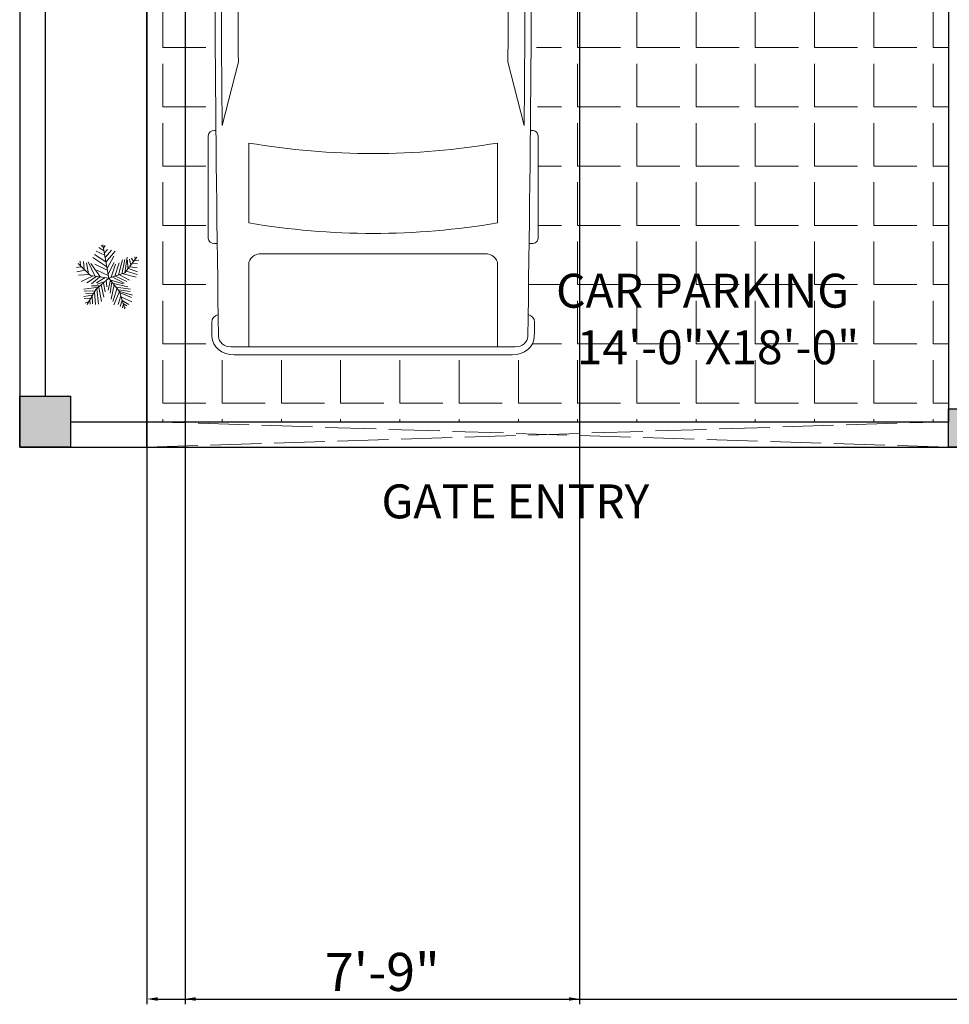
# Model space of a CAD drawing. Units: inches. Extents: x 889 to 1572, y 7262 to 8387.
# Tile 1 of 8: x 986 to 1205, y 7262 to 7495. Entities that reach past the tile are written whole.
import ezdxf

# ---------------------------------------------------------------- set-up
doc = ezdxf.new("R2010")
doc.units = ezdxf.units.IN
doc.linetypes.add('ACAD_ISO02W100', pattern=[15, 12, -3])
for name, color, linetype, lineweight in [('A-ANNO-DIMS', 2, 'Continuous', 18), ('A-ANNO-TEXT', 7, 'Continuous', 18), ('A-AREA-IDEN', 7, 'Continuous', 18), ('A-WALL', 7, 'Continuous', 35), ('C-SITE', 7, 'Continuous', 30), ('C-SITE-PATT', 252, 'Continuous', 13), ('C-VEHI', 8, 'Continuous', 18), ('L-PLNT', 94, 'Continuous', 13), ('L-PVMT-PATT', 252, 'Continuous', 13)]:
    doc.layers.add(name, color=color, linetype=linetype, lineweight=lineweight)
doc.layers.add('C-SITE-GATE', color=244, linetype='ACAD_ISO02W100', lineweight=18, true_color=0x991b1e)
doc.styles.get("Standard").update_dxf_attribs({"font": 'arial.ttf'})
doc.dimstyles.new('ISO-25', dxfattribs={"dimtxt": 9, "dimasz": 2.5, "dimexe": 1.25, "dimexo": 0.625, "dimtad": 1, "dimlunit": 3, "dimtxsty": 'Standard', "dimcen": 2.5, "dimadec": 0, "dimazin": 0, "dimtfac": 1, "dimtmove": 0, "dimatfit": 3, "dimfxl": 1, "dimarcsym": 0})

# ---------------------------------------------------------------- blocks, each defined once
blk = doc.blocks.new('*U21')
for p, q in [((21.10406751471477, 37.40863046792069), (21.10406751471477, 36.83230215753705)), ((46.55368679439944, 38.88847654282876), (22.35054758993934, 38.88847654282876)), ((47.80016686962392, 37.39011648242055), (47.80016686962392, 37.40863046792069)), ((135.4513231603356, 37.07354110333037), (135.4513231603356, 37.40863046792069)), ((136.6978032355602, 38.88847654282876), (160.90094244002, 38.88847654282867)), ((162.1474225152445, 37.40863046792049), (162.1474225152445, 36.77402019194128)), ((87.98532186932616, 31.87120872459877), (74.75900729854769, 35.92175679182955)), ((134.313356548143, 35.6043097713567), (119.2882629232503, 31.77757799177584)), ((186.4728846989705, -33.49860931502491), (186.4728846989718, 33.49860931502465)), ((188.3990091454065, -32.75868627757393), (188.3990091454077, 32.75868627757058)), ((70.0302824853563, 31.53613089391356), (86.40615155322342, 29.35124891408057)), ((138.4228833961707, 29.35124891408074), (157.2465674415997, 29.35124891408074)), ((186.4728846989718, 29.35124891408083), (167.0083537481071, 29.35124891408083)), ((164.515393597658, 26.39155676426461), (164.5153935976578, -26.39155676426503)), ((32.26591480791686, 11.62530558863241), (36.12873726252356, 17.16961494239206)), ((36.12873726252356, 17.16961494239206), (50.93891189819171, 17.16961494239206)), ((29.77279020470884, 9.505833383620029), (51.68362801571248, 9.505833383620029)), ((32.12291633764599, 9.505833383620029), (32.12291633764599, 11.15369945057711)), ((58.9167604809788, -10.77488335095668), (58.9167604809788, 10.77488335095617)), ((66.55009204259746, -10.5288681329018), (66.55009204259746, 10.52886813290129)), ((186.4728846989718, -10.5288681329018), (186.4728846989718, 10.52886813290129)), ((82.73706193978568, 8.496039918672748), (82.73706193978568, -8.49603991867258)), ((3.266462181856987, 6.128290093440767), (0.1022408397004821, 0.4060708604429806)), ((-4.43e-14, -2.558e-13), (51.68362801571248, -2.558e-13)), ((0.1022408397004821, -0.4060708604432933), (3.266462181856987, -6.128290093441194)), ((29.77279020470884, -9.50583338362054), (51.68362801571248, -9.50583338362054)), ((32.12291633764599, -9.50583338362054), (32.12291633764599, -11.15369945057762)), ((32.26591480791686, -11.62530558863292), (36.12873726252356, -17.16961494239257)), ((36.12873726252356, -17.16961494239257), (50.93891189819171, -17.16961494239257)), ((86.40615155322318, -29.35124891408145), (70.03028248535594, -31.53613089391442)), ((157.2465674415997, -29.35124891408117), (138.4228833961707, -29.35124891408126)), ((167.008353748107, -29.35124891408126), (186.4728846989707, -29.35124891408108)), ((87.98532186932607, -31.87120872459903), (74.7590072985476, -35.92175679182964)), ((134.3133565481428, -35.60430977135721), (119.2882629232503, -31.77757799177618)), ((21.10406751471477, -37.4086304679212), (21.10406751471477, -36.83230215753756)), ((135.4513231603355, -37.07354110333088), (135.4513231603355, -37.4086304679212)), ((162.1474225152445, -37.408630467921), (162.1474225152445, -36.77402019194179)), ((46.55368679439944, -38.88847654282927), (22.35054758993934, -38.88847654282927)), ((47.80016686962392, -37.39011648242107), (47.80016686962392, -37.4086304679212)), ((136.6978032355602, -38.88847654282927), (160.9009424400199, -38.88847654282918))]:
    blk.add_line(p, q)
for centre, major_axis, ratio, start_param, end_param in [((41.19115208863305, -490.8631038926156), (1.294e-13, 528.2339998381949), 0.8423038695439741, 0.0028100083536837, 0.0755983031096952), ((22.35054758993934, 37.40863046792072), (2.08e-14, -1.479846074908118), 0.842303869543976, 3.141592653589776, 4.712388980384677), ((64.48199294511879, -10555.61767587835), (1.907644e-10, 10593.02630634627), 0.842303869543847, -0.0133969486112073, 0.0027970409639888), ((46.55368679439944, 37.40863046792072), (2.2e-14, 1.479846074908118), 0.8423038695439758, -1.570796326794884, 1.73e-14), ((136.6978032355602, 37.40863046792072), (2.357e-13, -1.479846074908118), 0.842303869543976, 3.141592653589603, 4.712388980384554), ((160.90094244002, 37.40863046792052), (5.59e-14, 1.479846074908118), 0.842303869543976, -1.570796326794865, 4.44e-14), ((180.6280394947615, 35.8381667808375), (7.4e-14, 2.219769112362114), 0.8423038695439693, -0.0130174256259048, 1.249894140392862), ((64.48199294754608, -10556.35759891604), (1.349839377e-06, 10595.3130398087), 0.8423038681351469, -0.0133969484821159, -0.0130174254969711), ((183.9799245485216, 32.75868627756583), (8.56e-14, -5.246425615115243), 0.8423038695439737, 1.570796326795794, 3.128195704978164), ((266.0300214172791, -27.52442688366631), (1.966072e-10, 313.3077612809058), 0.8423038695435284, 1.367075990158062, 1.391760499156098), ((64.4819929449925, -10555.61767590795), (1.9177683e-09, -10591.54646030096), 0.8423038695482963, 3.133765086725325, 3.140440689641252), ((183.9799245485226, 33.49860931502124), (3e-16, -2.959692149816168), 0.8423038695439952, 1.570796326796048, 3.128195704978389), ((135.2911776514449, 5.387441675478555), (2.2715e-12, 81.77258453065997), 0.8423038695439563, 1.245306111696802, 1.507880129813836), ((95.78879860270445, -3666.353346297651), (1.949864e-10, -3698.236159209632), 0.8423038695446962, 3.134048706297306, 3.14409775411291), ((259.1750197310735, -27.52442688366614), (1.506617e-10, -305.3028914627677), 0.8423038695443789, 4.528606069860317, 4.561837674556238), ((37.47375371777758, -593.9621830607928), (6.21e-14, -623.32820996736), 0.8423038695439826, 3.09604606856106, 3.200911180495224), ((134.4003789125686, 5.387441675477674), (4.276e-13, -89.7774543484738), 0.84230386954398, 4.44948196380473, 4.652344057257214), ((149.595361812917, 2.799442537139299), (8.561e-13, -79.57966406425402), 0.842303869543983, 4.372215489277867, 4.640744122441986), ((17.08207736189386, -1.421e-13), (6.87e-14, 147.0179238898305), 0.8423038695439764, 4.511394369635731, 4.913383591133647), ((35.90576140732288, -1.421e-13), (6.87e-14, 147.0179238898305), 0.8423038695439764, 4.511394369635731, 4.913383591133647), ((167.0083537481071, 26.39155676426464), (1.394e-13, 2.959692149816236), 0.842303869543976, 5.55e-14, 1.57079632679492), ((-204.4946649195746, 52.39684969293512), (4.12053e-11, -250.9602162198571), 0.8423038695441164, 1.385369446298923, 1.434372047871027), ((13.03653510440275, 17.00972444508943), (1.2303e-12, 27.41599049210566), 0.8423038695439277, 4.435146050259648, 4.718221029521873), ((14.20086229321332, 17.00972444508943), (1.2303e-12, 27.41599049210566), 0.8423038695439277, 4.435146050259648, 4.718221029521873), ((50.7902773840875, 13.33772416300607), (6.340077547122382, -0.356608581037027), 0.6038335755719145, -1.39555193967809, 1.581314658479915), ((32.74615637525823, 11.15369945057713), (1.313e-13, 0.7399230374541176), 0.8423038695439091, 0.8797135699495516, 1.570796326795045), ((29.77279020470884, -46.66302566589627), (5.12e-14, 56.16885904951626), 0.842303869543976, 7e-16, 0.5903187773915901), ((0.6232400376122422, -1.421e-13), (1e-16, -0.7399230374541245), 0.842303869543842, 4.131459131953847, 5.293318828815531), ((29.77279020470884, 46.66302566589578), (4.004e-13, 56.16885904951626), 0.8423038695439734, 2.55127387619821, 3.141592653589801), ((-204.4946649195746, -52.39684969293552), (4.02945e-11, 250.9602162198562), 0.8423038695441192, -1.43437204787103, -1.385369446298926), ((149.5953618129329, -2.799442537137565), (4.0897e-12, -79.57966406427697), 0.8423038695439419, -1.499151468852248, -1.230622835688196), ((32.74615637525823, -11.1536994505777), (1.3e-13, -0.7399230374541176), 0.8423038695439093, 4.712388980384541, 5.403471737230034), ((13.03653510440275, -17.00972444508983), (1.2568e-12, -27.41599049210552), 0.8423038695439318, 1.564964277657711, 1.848039256919935), ((14.20086229321332, -17.00972444508983), (1.2568e-12, -27.41599049210552), 0.8423038695439318, 1.564964277657711, 1.848039256919935), ((134.4003789125684, -5.387441675478584), (4.2949e-12, -89.77745434847827), 0.8423038695439354, -1.510751403667474, -1.307889310215002), ((135.2911776514465, -5.387441675480715), (3.2038e-12, -81.77258453066244), 0.8423038695439492, -1.50788012981387, -1.245306111696839), ((259.1750197310694, 27.52442688365929), (1.08535e-11, 305.3028914629043), 0.8423038695439974, 1.721347632622872, 1.754579237318777), ((167.008353748107, -26.39155676426503), (1.02e-14, -2.959692149816192), 0.8423038695439885, 4.712388980384686, 6.283185307179581), ((266.0300214172791, 27.52442688366566), (8.75241e-11, 313.3077612806533), 0.8423038695441819, 1.749832154434603, 1.774516663432659), ((37.47375371777847, 593.9621830607904), (1.1693e-12, -623.3282099673584), 0.8423038695439528, -0.0593185269054384, 0.0455465850287298), ((95.78879860271888, 3666.35334629765), (1.637818e-10, -3698.236159209629), 0.8423038695447546, -0.0025051005232382, 0.007543947292366), ((183.9799245485216, -33.4986093150211), (9.3e-15, 2.959692149816141), 0.8423038695439732, 3.154989602201626, 4.71238898038339), ((183.9799245485177, -32.7586862775633), (2.428e-13, -5.246425615118353), 0.8423038695439808, 0.0133969486110846, 1.570796326792831), ((41.19115208863322, 490.8631038926152), (1.37757e-11, -528.2339998381949), 0.8423038695440652, -0.0755983031097181, -0.0028100083537155), ((64.48199294495228, 10555.61767590795), (6.117947e-10, 10593.02630637587), 0.8423038695458146, 3.138795612625926, 3.154989602201039), ((64.48199294503607, 10555.61767590793), (1.6049794e-09, -10591.54646030094), 0.8423038695397146, 0.0011519639481523, 0.0078275668641468), ((180.6280394947581, -35.83816678083949), (2.274e-13, -2.219769112363032), 0.8423038695439803, -1.249894138785958, 0.0130174256254374), ((22.35054758993934, -37.40863046792117), (2.2e-14, 1.479846074908118), 0.8423038695439758, 1.570796326794908, 3.14159265358981), ((46.55368679439944, -37.40863046792117), (2.08e-14, -1.479846074908118), 0.842303869543976, -1.69e-14, 1.570796326794884), ((136.6978032355602, -37.40863046792109), (1.56e-14, -1.479846074908162), 0.8423038695440105, -1.570796326794875, -1.27e-14), ((160.9009424400199, -37.408630467921), (1.969e-13, 1.479846074908162), 0.8423038695440109, 3.141592653589951, 4.712388980384771), ((64.48199294197605, 10556.3575989598), (9.365289701e-07, 10595.31303985772), 0.8423038705260315, 3.154610079306566, 3.154989602290631)]:
    blk.add_ellipse(centre, major_axis=major_axis, ratio=ratio, start_param=start_param, end_param=end_param)
at = {"extrusion": (0, 0, -1)}
blk.add_ellipse((50.7902773840875, -13.33772416300655), major_axis=(6.340077547122382, 0.3566085810370246), ratio=0.6038335755719145, start_param=-1.39555193967809, end_param=1.581314658479915, dxfattribs=at)
blk = doc.blocks.new('*U15')
for p, q in [((-8.736999999999625, 47.13799999999969), (-17.06899999999996, 52.71100000000001)), ((-10.18600000000015, 53.63999999999987), (-13.08399999999983, 55.96199999999976)), ((0, 0), (-10.5, 57)), ((-9.098999999999705, 51.7819999999997), (-6.563000000000101, 55.96199999999976)), ((-3.665000000000418, 19.27299999999968), (-27.57400000000007, 35.52699999999982)), ((-5.114000000000032, 28.09699999999975), (-24.67599999999993, 40.63599999999996)), ((-7.28800000000001, 39.70699999999965), (-21.77800000000025, 46.67299999999977)), ((-7.65000000000009, 43.42299999999977), (-2.577999999999974, 49.45999999999981)), ((-5.838999999999941, 35.99199999999973), (4.666999999999916, 48.06699999999977)), ((-5.114000000000032, 27.63199999999983), (10.46300000000019, 46.67299999999977)), ((-2.940999999999803, 16.48599999999987), (8.652000000000044, 37.84999999999991)), ((27, 9), (48, 36)), ((27.12699999999995, 9.05600000000004), (31.11200000000008, 35.99199999999973)), ((38.71900000000005, 34.13399999999979), (41.97899999999981, 28.56099999999992)), ((44.15300000000025, 36.45599999999991), (45.23900000000003, 32.74099999999999)), ((-47.49800000000004, 19.73699999999962), (-55.83000000000038, 18.34399999999982)), ((-31.5, 4.5), (-52.5, 25.5)), ((-48.58500000000003, 21.13099999999986), (-49.30899999999974, 29.02600000000007)), ((-43.51299999999992, 28.56099999999992), (-42.42699999999968, 15.55799999999976)), ((-38.44199999999955, 26.23899999999981), (-34.81899999999996, 7.662999999999783)), ((-35.54399999999987, 28.09699999999975), (-24.31399999999985, 3.946999999999661)), ((-14.5329999999999, 2.089999999999918), (-30.83399999999983, 25.30999999999995)), ((-24.31399999999985, 23.91699999999969), (-2.940999999999803, 13.69999999999982)), ((-1.128999999999905, 6.733999999999923), (9.014000000000124, 26.70399999999995)), ((3.942000000000007, 1.625), (11.1869999999999, 24.38099999999986)), ((10.10100000000011, 3.482999999999719), (17.70800000000008, 26.23899999999981)), ((16.25900000000001, 5.804999999999836), (23.14199999999983, 31.34799999999973)), ((22.05499999999984, 7.197999999999865), (27.48900000000003, 32.27699999999982)), ((31.83600000000024, 30.88299999999981), (32.56100000000015, 16.48599999999987)), ((35.09600000000001, 32.74099999999999), (37.26999999999998, 22.52399999999989)), ((36.18300000000045, 19.73699999999962), (48.13699999999972, 17.87999999999988)), ((40.52999999999975, 25.77499999999986), (48.86200000000008, 24.846)), ((43.79100000000017, 29.95399999999995), (51.03600000000006, 30.88299999999981)), ((-40.61500000000023, 13.69999999999982), (-55.10500000000002, 10.91299999999978)), ((-33.37000000000035, 6.268999999999778), (-52.20699999999988, 5.339999999999918)), ((-28.29899999999998, 3.482999999999719), (-47.86000000000012, -5.805000000000063)), ((-21.41600000000017, 3.017999999999801), (-38.07899999999973, -8.128000000000384)), ((0, 0), (-31.5, 4.5)), ((-15.98199999999951, 2.089999999999918), (-30.11000000000013, -9.521000000000186)), ((0, 0), (-22.5, -19.5)), ((-6.563000000000101, 1.161000000000058), (-21.41600000000017, -8.128000000000384)), ((-20.69099999999981, 13.69999999999982), (-1.128999999999905, 4.875999999999976)), ((0, 0), (27, 9)), ((0, 0), (18, -22.5)), ((6.478000000000065, 1.625), (26.03999999999996, -8.592000000000326)), ((11.1869999999999, 3.482999999999719), (30.74900000000025, -5.805000000000063)), ((18.06999999999971, 5.804999999999836), (35.09600000000001, -3.483000000000174)), ((24.22899999999982, 7.662999999999783), (46.6880000000001, 1.625)), ((29.66199999999981, 12.30699999999979), (48.13699999999972, 6.268999999999778)), ((33.28499999999986, 16.48599999999987), (48.86200000000008, 10.91299999999978)), ((-17.43100000000004, -15.09400000000005), (-42.78899999999976, -18.80899999999997)), ((-15.2569999999996, -12.77200000000016), (-30.11000000000013, -12.77200000000016)), ((-6.563000000000101, -5.805000000000063), (-19.96699999999964, -9.985000000000127)), ((-17.06899999999996, -15.09400000000005), (-12.721, -40.17200000000025)), ((-13.44599999999991, -11.37800000000038), (-8.736999999999625, -32.74100000000021)), ((-9.460999999999785, -8.592000000000326), (-6.201000000000021, -23.4530000000002)), ((-4.751999999999952, -3.483000000000174), (-3.665000000000418, -14.62900000000013)), ((2.493000000000392, -3.019000000000005), (-1.490999999999985, -20.20200000000023)), ((1.769000000000232, -2.555000000000063), (24.22899999999982, -9.521000000000186)), ((5.028999999999996, -6.270000000000209), (2.131000000000312, -25.77500000000009)), ((9.014000000000124, -11.37800000000038), (3.579999999999927, -35.99200000000019)), ((7.564999999999599, -9.056000000000267), (32.19800000000032, -14.62900000000013)), ((12.27399999999988, -15.09400000000005), (36.9069999999997, -18.80899999999997)), ((-28.29899999999998, -29.02600000000007), (-42.78899999999976, -31.34800000000018)), ((-24.31399999999985, -21.59600000000023), (-42.42699999999968, -22.06000000000017)), ((-26.8489999999997, -26.24000000000001), (-40.25300000000015, -25.77500000000009)), ((-22.5, -19.5), (-37.5, -45)), ((-29.02300000000014, -30.88400000000002), (-27.93600000000015, -43.88700000000016)), ((-25.03800000000001, -23.91800000000035), (-22.86500000000024, -45.28100000000017)), ((-20.69099999999981, -18.34500000000003), (-17.79300000000012, -44.35200000000032)), ((14.08499999999958, -16.95100000000025), (6.478000000000065, -40.17200000000025)), ((18.06999999999971, -22.52400000000012), (8.289000000000215, -45.74500000000012)), ((20.24400000000014, -30.4190000000001), (15.89699999999993, -44.81600000000026)), ((16.25900000000001, -19.73800000000028), (36.18300000000045, -22.98900000000003)), ((18, -22.5), (27, -52.5)), ((18.43300000000045, -22.52400000000012), (40.52999999999975, -29.02600000000007)), ((19.1569999999997, -25.31100000000015), (38.71900000000005, -33.20600000000013)), ((21.33100000000013, -32.74100000000021), (39.08100000000013, -40.63600000000019)), ((-30.83399999999983, -34.13499999999999), (-42.42699999999968, -35.52800000000025)), ((-34.45699999999988, -39.70800000000031), (-40.97800000000006, -42.49400000000014)), ((-32.64600000000019, -36.92100000000005), (-31.92099999999982, -44.35200000000032)), ((22.77999999999975, -37.85000000000014), (19.51900000000023, -48.53200000000015)), ((22.77999999999975, -38.31400000000008), (34.37199999999985, -44.81600000000026)), ((24.59100000000035, -45.74500000000012), (23.14199999999983, -50.85400000000004)), ((24.59100000000035, -43.42300000000022), (30.74900000000025, -47.60300000000029)), ((26.76400000000012, -49.92500000000018), (28.21300000000019, -50.85400000000004))]:
    blk.add_line(p, q)
blk = doc.blocks.new('*D69')
at = {"layer": 'A-ANNO-DIMS', "color": 0, "lineweight": -2, "transparency": 16777216}
for p, q in [((1016.048608, 7615.106231), (1016.048608, 7262.354215000001)), ((1436.048608, 7582.106231), (1436.048608, 7262.354215000001)), ((1018.548608, 7263.604215), (1433.548608, 7263.604215))]:
    blk.add_line(p, q, dxfattribs=at)
at = {"layer": 'A-ANNO-DIMS', "color": 0, "transparency": 16777216}
for points in [[(1018.548608, 7264.020881666667), (1018.548608, 7263.187548333333), (1016.048608, 7263.604215)], [(1433.548608, 7264.020881666667), (1433.548608, 7263.187548333333), (1436.048608, 7263.604215)]]:
    blk.add_solid(points, dxfattribs=at)
at = {"layer": 'Defpoints', "color": 0, "transparency": 16777216}
for p in [(1016.048608, 7615.731230999999), (1436.048608, 7582.731231), (1436.048608, 7263.604215)]:
    blk.add_point(p, dxfattribs=at)
at = {"layer": 'A-ANNO-DIMS', "color": 0, "transparency": 16777216, "insert": (1226.048608, 7268.827441466576), "char_height": 9, "attachment_point": 5}
blk.add_mtext('35\'-0"', dxfattribs=at)
blk = doc.blocks.new('*D76')
at = {"layer": 'A-ANNO-DIMS', "color": 0, "lineweight": -2, "transparency": 16777216}
for p, q in [((1025.048608, 7774.106231000001), (1025.048608, 7262.354215000001)), ((1118.048608, 7774.106231000001), (1118.048608, 7262.354215000001)), ((1027.548608, 7263.604215), (1115.548608, 7263.604215))]:
    blk.add_line(p, q, dxfattribs=at)
at = {"layer": 'A-ANNO-DIMS', "color": 0, "transparency": 16777216}
for points in [[(1027.548608, 7264.020881666667), (1027.548608, 7263.187548333333), (1025.048608, 7263.604215)], [(1115.548608, 7264.020881666667), (1115.548608, 7263.187548333333), (1118.048608, 7263.604215)]]:
    blk.add_solid(points, dxfattribs=at)
at = {"layer": 'Defpoints', "color": 0, "transparency": 16777216}
for p in [(1025.048608, 7774.731231), (1118.048608, 7774.731231), (1118.048608, 7263.604215)]:
    blk.add_point(p, dxfattribs=at)
at = {"layer": 'A-ANNO-DIMS', "color": 0, "transparency": 16777216, "insert": (1071.548608, 7268.824371889495), "char_height": 9, "attachment_point": 5}
blk.add_mtext('7\'-9"', dxfattribs=at)

msp = doc.modelspace()

# ---------------------------------------------------------------- hatches: boundary and pattern name
at = {"layer": 'C-SITE-PATT'}
h = msp.add_hatch(color=256, dxfattribs=at)
h.dxf.hatch_style = 1
h.paths.add_polyline_path([(1214.048608413347, 7402.731230872603), (1205.048608413347, 7402.731230872603), (1205.048608413347, 7393.731230872605), (1214.048608413347, 7393.731230872605)])
h.paths.add_polyline_path([(1265.481018479948, 7402.731230872602), (1256.481018479948, 7402.731230872602), (1256.481018479948, 7393.731230872602), (1265.481018479948, 7393.731230872602)])
h.paths.add_polyline_path([(998.0486084133516, 7405.731230872598), (986.0486084133516, 7405.731230872598), (986.0486084133516, 7393.731230872599), (998.0486084133516, 7393.731230872599)])
at = {"layer": 'L-PVMT-PATT'}
h = msp.add_hatch(dxfattribs=at)
h.set_pattern_fill('ANGLE', color=256, scale=2)
h.set_pattern_definition([(0, (0, 0), (0, 13.97), [10.16, -3.81]), (90, (0, 0), (-13.97, 9e-16), [10.16, -3.81])])
h.paths.add_polyline_path([(1205.048608413351, 7555.446171834415), (1204.522810014118, 7555.264684699134), (1205.048608413351, 7555.910703335377), (1205.048608413352, 7557.193763035785), (1204.375295363129, 7557.060960744141), (1205.048608413352, 7557.600559978721), (1205.048608413352, 7559.617877481), (1204.375295363129, 7559.330134346581), (1204.006412068125, 7559.046511813157), (1204.08026606115, 7559.708297724476), (1205.048608413352, 7561.087614386948), (1205.048608413352, 7561.676628270497), (1205.03901462505, 7561.693848793495), (1204.227780712139, 7562.166553015865), (1205.048608413352, 7562.166553015865), (1205.048608413352, 7565.277573844389), (1205.03901462505, 7565.286594218571), (1205.048608413352, 7565.286594218571), (1205.048608413352, 7578.731230872603), (1159.234402724352, 7578.731230872605), (1159.234402724352, 7578.363210835082, -0.1960004452144572), (1159.622195581334, 7577.411949376209, -1.441243748687975), (1157.234402724352, 7578.304265881411), (1157.234402724352, 7615.731230872604), (1016.048608413352, 7615.731230872608), (1016.048608413352, 7399.731230872607), (1022.048608413351, 7399.731230872605), (1205.048608413347, 7399.731230872603), (1205.048608413347, 7402.731230872603)])
edge = h.paths.add_edge_path(flags=16)
edge.add_ellipse((-9486.215667076898, 7539.371191098851), major_axis=(10593.02630634627, 3.017206e-10), ratio=0.8423038695454096, start_angle=-0.38386677879407216, end_angle=0.09022908859270728, ccw=False)
edge.add_ellipse((1106.81063926937, 7467.155380808408), major_axis=(1.479846074908209, 2.4527e-12), ratio=0.8423038695436039, start_angle=-9.487166607868858e-11, end_angle=89.99999999990501, ccw=False)
edge.add_line((1108.290485344278, 7467.155380808408), (1108.290485344278, 7442.952241603949))
edge.add_ellipse((1106.81063926937, 7442.952241603949), major_axis=(-1.479846074908209, 2.4527e-12), ratio=0.8423038695436041, start_angle=90.00000000009499, end_angle=180.0000000000949, ccw=False)
edge.add_line((1106.81063926937, 7441.705761528725), (1106.176028993391, 7441.705761528725))
edge.add_ellipse((-9486.215667076898, 7539.371191098851), major_axis=(10593.02630634627, 3.017206e-10), ratio=0.8423038695454096, start_angle=-0.6186431963208179, end_angle=-0.5282714718196075, ccw=False)
edge.add_ellipse((1105.240175582287, 7423.225144549206), major_axis=(2.219769112362271, 3.512e-12), ratio=0.8423038695437586, start_angle=-0.6282372162759771, end_angle=68.464756600913, ccw=False)
edge.add_ellipse((-9486.955590114589, 7539.371191096425), major_axis=(-10595.31303979869, 5.7334850558e-06), ratio=0.8423038635969176, start_angle=179.3534459339559, end_angle=179.3717628147891, ccw=False)
edge.add_ellipse((1102.160695079015, 7419.873259495446), major_axis=(-5.246425615115091, 6.131e-13), ratio=0.8423038695439657, start_angle=90.00000000006861, end_angle=179.3534459029308, ccw=False)
edge.add_line((1102.16069507902, 7415.45417489856), (1036.643322523875, 7415.454174898562))
edge.add_ellipse((1036.643322523886, 7419.87325949545), major_axis=(5.246425615118246, 3.3658e-12), ratio=0.8423038695439792, start_angle=180.6465540970289, end_angle=269.9999999998247, ccw=False)
edge.add_ellipse((11625.75960776125, 7539.371191101991), major_axis=(-10595.31303986147, 2.5904085676e-06), ratio=0.8423038722500887, start_angle=0.6282372302511021, end_angle=0.6465541110841855, ccw=False)
edge.add_ellipse((1033.56384202061, 7423.225144549211), major_axis=(2.219769112362928, 1.9515e-12), ratio=0.8423038695441785, start_angle=111.5352435039708, end_angle=180.6282372161348, ccw=False)
edge.add_ellipse((11625.0196847094, 7539.371191099013), major_axis=(-10593.02630637587, 5.863276e-10), ratio=0.8423038695454017, start_angle=0.528271471820517, end_angle=0.646554097064211, ccw=False)
edge.add_line((1032.627988609511, 7441.705761528725), (1031.993378333528, 7441.705761528725))
edge.add_ellipse((1031.993378333528, 7442.952241603949), major_axis=(1.479846074908209, 2.4527e-12), ratio=0.8423038695436039, start_angle=179.999999999905, end_angle=269.999999999905, ccw=False)
edge.add_line((1030.51353225862, 7442.952241603949), (1030.51353225862, 7467.155380808408))
edge.add_ellipse((1031.993378333528, 7467.155380808408), major_axis=(-1.479846074908209, 2.4527e-12), ratio=0.8423038695436041, start_angle=-89.99999999990501, end_angle=9.498535291641019e-11, ccw=False)
edge.add_ellipse((11625.0196847094, 7539.371191099013), major_axis=(-10593.02630637587, 5.863276e-10), ratio=0.8423038695454017, start_angle=-0.0902290885899788, end_angle=0.38386677879549325, ccw=False)
edge.add_ellipse((1031.993378333528, 7557.299497249569), major_axis=(-1.479846074907982, 9.504e-13), ratio=0.8423038695443477, start_angle=3.6777692002942786e-11, end_angle=90.00000000003672, ccw=False)
edge.add_line((1030.51353225862, 7557.299497249569), (1030.51353225862, 7581.502636454029))
edge.add_ellipse((1031.993378333528, 7581.502636454029), major_axis=(-1.479846074907982, 2.1793e-12), ratio=0.8423038695437334, start_angle=-89.99999999991559, end_angle=8.44124770082999e-11, ccw=False)
edge.add_line((1031.993378333528, 7582.749116529253), (1032.569706643912, 7582.749116529253))
edge.add_ellipse((1560.265112694065, 7562.662031955335), major_axis=(528.2339998381949, 5.3105e-12), ratio=0.8423038695440039, start_angle=176.3495724143003, end_angle=177.8200496863542, ccw=False)
edge.add_ellipse((1096.926435685115, 7337.82316262669), major_axis=(-313.3077612789123, 2.032944e-09), ratio=0.84230386954869, start_angle=-77.87403444734417, end_angle=-76.21947101013029, ccw=False)
edge.add_ellipse((1096.926435685109, 7344.678164312899), major_axis=(-305.3028914625973, 2.877231e-10), ratio=0.842303869544824, start_angle=-79.79046100280272, end_angle=-77.55537270650188, ccw=False)
edge.add_ellipse((1017.005159108514, 7808.347848963542), major_axis=(250.9602162202823, 3.689106e-10), ratio=0.8423038695427255, start_angle=-80.7434339928827, end_angle=-77.44506735594696)
edge.add_line((1063.273718708008, 7600.586721862112), (1069.402008801449, 7603.975488617634))
edge.add_line((1069.402008801449, 7603.975488617634), (1075.53029889489, 7600.586721862112))
edge.add_ellipse((1121.798858494384, 7808.347848963542), major_axis=(-250.9602162202835, 3.684091e-10), ratio=0.8423038695427219, start_angle=77.44506735594675, end_angle=80.74343399288247)
edge.add_ellipse((1041.877581917783, 7344.678164312894), major_axis=(305.3028914626093, 3.003322e-10), ratio=0.842303869544806, start_angle=77.55537270649842, end_angle=79.79046100279919, ccw=False)
edge.add_ellipse((1041.877581917783, 7337.82316262669), major_axis=(313.3077612789065, 2.0431705e-09), ratio=0.8423038695487045, start_angle=76.21947101012842, end_angle=77.87403444734218, ccw=False)
edge.add_ellipse((578.5389049088338, 7562.662031955335), major_axis=(-528.2339998381949, 1.51629e-11), ratio=0.8423038695441082, start_angle=182.1799503136469, end_angle=183.6504275857008, ccw=False)
edge.add_line((1106.234310958986, 7582.749116529253), (1106.81063926937, 7582.749116529253))
edge.add_ellipse((1106.81063926937, 7581.502636454029), major_axis=(1.479846074908209, 2.4524e-12), ratio=0.8423038695436039, start_angle=-9.487166607868858e-11, end_angle=89.99999999989461, ccw=False)
edge.add_line((1108.290485344278, 7581.502636454029), (1108.290485344278, 7557.299497249569))
edge.add_ellipse((1106.81063926937, 7557.299497249569), major_axis=(1.479846074908209, 6.78e-13), ratio=0.8423038695442183, start_angle=269.99999999997374, end_angle=359.9999999999738, ccw=False)
edge = h.paths.add_edge_path(flags=0)
edge.add_ellipse((-9486.215667106499, 7539.371191098978), major_axis=(10591.54646030096, 1.2635629e-09), ratio=0.8423038695462665, start_angle=-0.3777641939166756, end_angle=-0.055594313506105664, ccw=False)
edge.add_line((1105.006318572806, 7469.539827495825), (1101.179586793223, 7484.564921120725))
edge.add_ellipse((-2596.951337496201, 7508.064385441264), major_axis=(3698.23615920963, 2.129104e-10), ratio=0.8423038695460041, start_angle=-0.3640763488936447, end_angle=0.1208973690293594)
edge.add_line((1101.273217526047, 7515.867862174639), (1105.323765593278, 7529.094176745418))
edge = h.paths.add_edge_path(flags=0)
edge.add_line((1100.938139695363, 7533.822901558612), (1098.75325771553, 7517.447032490746))
edge.add_ellipse((1072.201451338588, 7454.257822231051), major_axis=(-79.57966406428197, 3.36667e-11), ratio=0.8423038695436982, start_angle=247.2080851224342, end_angle=265.1299304028885)
edge.add_line((1077.898048720122, 7521.116122104183), (1060.905968882777, 7521.116122104183))
edge.add_ellipse((1066.602566264312, 7454.257822231035), major_axis=(79.57966406429925, 3.47446e-11), ratio=0.842303869543722, start_angle=94.87006959711071, end_angle=112.7919148775615)
edge.add_line((1040.050759887368, 7517.447032490746), (1037.865877907535, 7533.822901558612))
edge.add_ellipse((1064.014567125969, 7468.562006392521), major_axis=(81.77258453066123, 3.0009e-12), ratio=0.8423038695439617, start_angle=94.27742096305201, end_angle=111.8349537967062, ccw=False)
edge.add_line((1058.873140668548, 7537.30309200137), (1079.930876934351, 7537.30309200137))
edge.add_ellipse((1074.789450476928, 7468.562006392524), major_axis=(81.77258453065926, 1.3305e-12), ratio=0.8423038695439597, start_angle=68.16504620328942, end_angle=85.7225790369435, ccw=False)
edge = h.paths.add_edge_path(flags=0)
edge.add_ellipse((1082.739732964455, 7553.062906659881), major_axis=(0.3566085810348156, 6.340077547122254), ratio=0.6038335755719637, start_angle=106.3425919542708, end_angle=270.9979857249622, ccw=False)
edge.add_line((1078.907842185069, 7552.169556028257), (1078.907842185069, 7574.080393839259))
edge.add_ellipse((1022.738983135553, 7574.080393839259), major_axis=(-56.16885904951628, 2.3357e-12), ratio=0.8423038695439936, start_angle=180.0000000000023, end_angle=209.4385695979816)
edge.add_ellipse((1116.065034467345, 7574.080393839259), major_axis=(56.16885904951618, 2.2359e-12), ratio=0.8423038695439938, start_angle=150.5614304020184, end_angle=179.9999999999977)
edge.add_line((1059.896175417829, 7574.08039383926), (1059.896175417829, 7552.169556028257))
edge.add_ellipse((1056.064284638443, 7553.062906659881), major_axis=(-0.3566085810390883, 6.340077547122437), ratio=0.6038335755718836, start_angle=89.00201427499962, end_angle=253.6574080456915, ccw=False)
edge.add_line((1052.232393859057, 7552.914272145777), (1052.232393859057, 7567.724446781444))
edge.add_line((1052.232393859057, 7567.724446781444), (1057.981948927734, 7571.730267706323))
edge.add_line((1057.981948927734, 7571.730267706323), (1059.896175417829, 7571.730267706323))
edge.add_line((1059.896175417829, 7571.730267706323), (1059.896175417829, 7574.08039383926))
edge.add_ellipse((1116.065034467345, 7574.080393839259), major_axis=(56.16885904951618, 2.2359e-12), ratio=0.8423038695439938, start_angle=150.5614304020184, end_angle=179.9999999999977, ccw=False)
edge.add_ellipse((1022.738983135553, 7574.080393839259), major_axis=(-56.16885904951628, 2.3357e-12), ratio=0.8423038695439936, start_angle=180.0000000000024, end_angle=209.4385695979817, ccw=False)
edge.add_line((1078.907842185069, 7574.080393839259), (1078.907842185069, 7571.730267706323))
edge.add_line((1078.907842185069, 7571.730267706323), (1080.822068675164, 7571.730267706323))
edge.add_line((1080.822068675164, 7571.730267706323), (1086.571623743841, 7567.724446781444))
edge.add_line((1086.571623743841, 7567.724446781444), (1086.571623743841, 7552.914272145774))
edge = h.paths.add_edge_path(flags=0)
edge.add_line((1098.75325771553, 7465.430300647797), (1098.75325771553, 7446.606616602368))
edge.add_ellipse((1069.402008801449, 7567.947422636645), major_axis=(-147.017923889832, 1.396e-13), ratio=0.8423038695439693, start_angle=76.4018653097695, end_angle=103.59813469023061, ccw=False)
edge.add_line((1040.050759887368, 7446.606616602368), (1040.050759887368, 7465.430300647797))
edge.add_ellipse((1069.402008801449, 7586.771106682075), major_axis=(-147.017923889832, 1.396e-13), ratio=0.8423038695439693, start_angle=76.4018653097695, end_angle=103.5981346902306)
edge = h.paths.add_edge_path(flags=0)
edge.add_ellipse((1095.793565565714, 7436.844830295861), major_axis=(-2.959692149816191, 1.9947e-12), ratio=0.842303869543976, start_angle=180.0000000000387, end_angle=270.0000000000386, ccw=False)
edge.add_line((1098.75325771553, 7436.844830295861), (1098.75325771553, 7417.380299344997))
edge.add_line((1098.75325771553, 7417.380299344997), (1040.050759887368, 7417.380299344998))
edge.add_line((1040.050759887368, 7417.380299344998), (1040.050759887368, 7436.844830295861))
edge.add_ellipse((1043.010452037184, 7436.844830295861), major_axis=(2.959692149816192, 1.9928e-12), ratio=0.8423038695439758, start_angle=89.9999999999614, end_angle=179.9999999999614, ccw=False)
edge.add_line((1043.010452037184, 7439.337790446311), (1095.793565565714, 7439.337790446311))
edge = h.paths.add_edge_path(flags=0)
edge.add_ellipse((4735.755355099098, 7508.064385441248), major_axis=(-3698.236159209629, 1.078002e-10), ratio=0.8423038695486287, start_angle=-0.1208973690313006, end_angle=0.3640763488917358)
edge.add_line((1037.624430809674, 7484.564921120725), (1033.797699030094, 7469.539827495835))
edge.add_ellipse((11625.01968470938, 7539.371191098929), major_axis=(10591.54646030094, 2.5735131e-09), ratio=0.8423038695346576, start_angle=180.0555943134852, end_angle=180.3777641938957, ccw=False)
edge.add_line((1033.480252009621, 7529.094176745418), (1037.530800076852, 7515.867862174644))
h.paths.add_polyline_path([(1109.981626785864, 7408.740466663437), (1190.985719555305, 7408.740466663437), (1190.985719555305, 7438.592217459254), (1109.981626785864, 7438.592217459254)], flags=24)

# ---------------------------------------------------------------- linework, layer by layer
at = {"layer": 'A-WALL'}
msp.add_line((1016.048608413352, 8272.731230872607), (1016.048608413352, 7393.731230872607), dxfattribs=at)
at = {"layer": 'C-SITE'}
for p, q in [((986.0486084133516, 8272.731230872607), (986.0486084133516, 7393.731230872607)), ((992.0486084133518, 8272.731230872607), (992.0486084133518, 7405.731230872598)), ((1205.048608413352, 7582.731230872609), (1205.048608413347, 7399.731230872605)), ((998.0486084133516, 7399.731230872608), (1022.048608413351, 7399.731230872605)), ((1022.048608413351, 7399.731230872609), (1205.048608413347, 7399.731230872603)), ((986.0486084133516, 7393.731230872607), (1466.048608413352, 7393.731230872599))]:
    msp.add_line(p, q, dxfattribs=at)
for points in [[(986.0486084133516, 7405.731230872598), (998.0486084133516, 7405.731230872598), (998.0486084133516, 7393.731230872599), (986.0486084133516, 7393.731230872599)], [(1205.048608413347, 7402.731230872603), (1214.048608413347, 7402.731230872603), (1214.048608413347, 7393.731230872605), (1205.048608413347, 7393.731230872605)]]:
    msp.add_lwpolyline(points, close=True, dxfattribs=at)
at = {"layer": 'C-SITE-GATE'}
for p, q in [((1016.048608413352, 7393.731230872607), (1205.048608413347, 7399.731230872603)), ((1205.048608413347, 7393.731230872605), (1016.048608413352, 7399.731230872607))]:
    msp.add_line(p, q, dxfattribs=at)

# ---------------------------------------------------------------- block references
at = {"layer": 'C-VEHI', "rotation": 270}
msp.add_blockref('*U21', (1069.402008801449, 7603.853184043969), dxfattribs=at)
at = {"layer": 'L-PLNT', "xscale": 0.137481440781912, "yscale": 0.137481440781912, "zscale": 0.137481440781912}
msp.add_blockref('*U15', (1007.09533939139, 7433.555527877068), dxfattribs=at)

# ---------------------------------------------------------------- texts
at = {"layer": 'A-ANNO-TEXT', "insert": (1071.356489634992, 7384.935022649829), "char_height": 8, "attachment_point": 1}
msp.add_mtext_dynamic_manual_height_columns('GATE ENTRY', width=76.77495777546574, gutter_width=12.5, heights=[0], dxfattribs=at)
at = {"layer": 'A-AREA-IDEN', "insert": (1112.538243429793, 7434.611317049976), "char_height": 8, "attachment_point": 1}
msp.add_mtext_dynamic_manual_height_columns('CAR PARKING\\P  14\'-0"X18\'-0"', width=76.77495777546574, gutter_width=12.5, heights=[0], dxfattribs=at)

# ---------------------------------------------------------------- dimensions: what is measured, and where the dimension line sits
at = {"layer": 'A-ANNO-DIMS'}
for base, p1, p2, picture, middle in [((1118.048608, 7263.604215), (1025.048608, 7774.731231), (1118.048608, 7774.731231), '*D76', (1071.548608, 7268.824371889495)), ((1436.048608, 7263.604215), (1016.048608, 7615.731230999999), (1436.048608, 7582.731231), '*D69', (1226.048608, 7268.827441466576))]:
    dim = msp.add_linear_dim(base=base, p1=p1, p2=p2, dimstyle='ISO-25', override={"dimdec": 1, "dimlfac": 1, "dimrnd": 0, "dimzin": 1, "dimdsep": 46, "dimlunit": 4, "dimfrac": 2}, dxfattribs=at)
    dim.commit()
    dim.dimension.update_dxf_attribs({"geometry": picture, "text_midpoint": middle})

doc.saveas('drawing.dxf')
